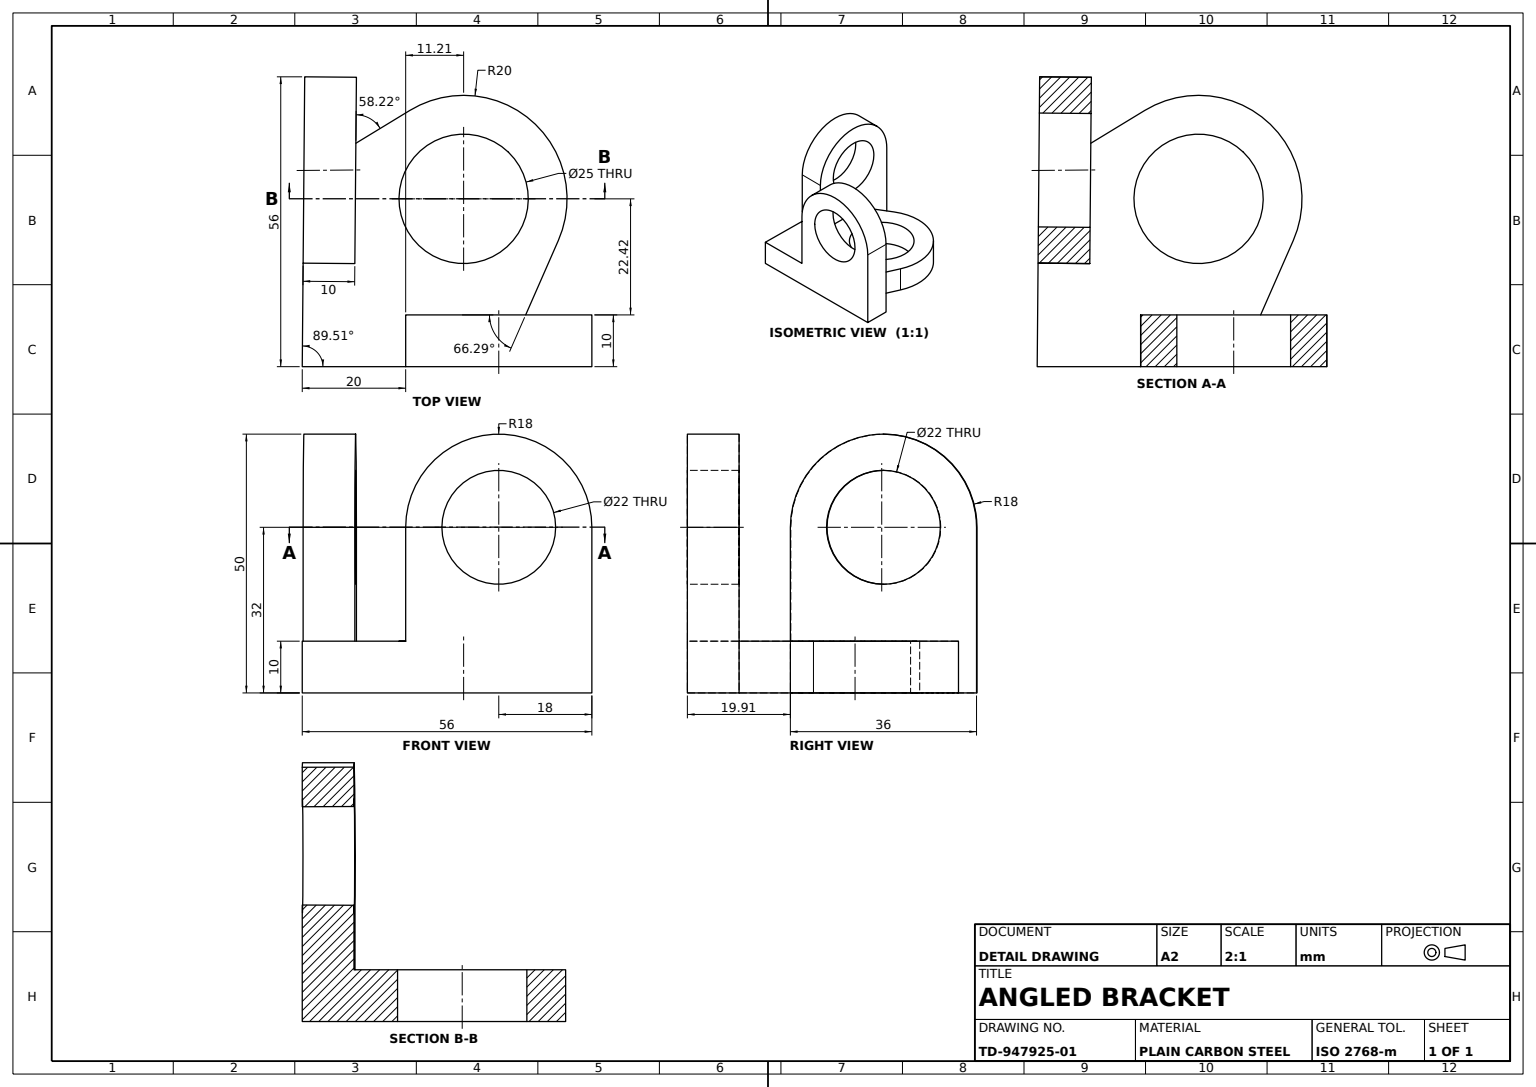
SolidWorks part; units mm, degrees
material "Plain Carbon Steel"
ref_plane "Front Plane" through (0, 0, 0) normal (0, 0, 1) x (1, 0, 0)
ref_plane "Top Plane" through (0, 0, 0) normal (0, 1, 0) x (1, 0, 0)
ref_plane "Right Plane" through (0, 0, 0) normal (1, 0, 0) x (0, 0, -1)
sketch "Base Plate Sketch" plane through (0, 0, 0) normal (0, 1, 0) x (1, 0, 0)
  line L0 (-19.3362, -21.1719) -> (-25.4663, -44.3681)
  line L1 (18.7702, -19.377) -> (27.9636, -44.3681)
  line L2 (-25.4663, -44.3681) -> (0, -71.2819)
  line L3 (0, -71.2819) -> (27.9636, -44.3681)
  arc A0 (18.7702, -19.377) -> (-19.3362, -21.1719) centre (0, -26.2819) ccw
  circle A1 centre (0, -26.2819) radius 12.5
  dimension "D1" = 40
  dimension "D2" = 25
  dimension "D5" = 26.2819
  dimension "D3" = 35
  dimension "D4" = 45
  dimension "D6" = 18.0862
  dimension "D7" = 25.4663
extrude "Base Plate" add sketch "Base Plate Sketch" along normal blind 10
ref_plane "Lug 1 Plane" through (35.6149, 0, 37.0041) normal (0.6935, 0, 0.7205) x (0.7205, 0, -0.6935)
sketch "Lug 1 Sketch" plane through (35.6149, 0, 37.0041) normal (0.6935, 0, 0.7205) x (0.7205, 0, -0.6935)
  line L0 (-29.4306, 10) -> (-29.4306, 32)
  line L1 (-49.4306, 10) -> (-10.6193, 10) construction
  line L3 (-10.6193, 10) -> (0.087, 10) construction
  line L4 (6.5694, 10) -> (6.5694, 32)
  line L5 (-49.4306, 10) -> (-49.4306, 0) construction
  line L6 (-49.4306, 0) -> (-10.6193, 0) construction
  line L9 (-29.4306, 10) -> (-29.4306, 0)
  line L10 (-29.4306, 0) -> (6.5694, 0)
  line L11 (6.5694, 10) -> (6.5694, 0)
  arc A0 (6.5694, 32) -> (-29.4306, 32) centre (-11.4306, 32) ccw
  circle A1 centre (-11.4306, 32) radius 11
  dimension "D4" = 36
  dimension "D5" = 22
  dimension "D1" = 20
  dimension "D2" = 32
  dimension "D3" = 36
  dimension "D6" = 18
  dimension "D7" = 10
extrude "Lug 1" add sketch "Lug 1 Sketch" against normal blind 10
ref_plane "Lug 2 Plane" through (-35.5865, 0, 33.6726) normal (-0.7264, 0, 0.6873) x (0.6873, 0, 0.7264)
sketch "Lug 2 Sketch" plane through (-35.5865, 0, 33.6726) normal (-0.7264, 0, 0.6873) x (0.6873, 0, 0.7264)
  line L0 (31.7771, 32) -> (31.7771, 0)
  line L2 (14.7246, 0) -> (51.7771, 0) construction
  line L3 (31.7771, 0) -> (-4.2229, 0)
  line L4 (2.0888, 0) -> (14.7246, 0) construction
  line L5 (-4.2229, 0) -> (-4.2229, 32)
  line L6 (51.7771, 10) -> (51.7771, 0) construction
  circle A0 centre (13.7771, 32) radius 11
  arc A1 (31.7771, 32) -> (-4.2229, 32) centre (13.7771, 32) ccw
  dimension "D1" = 36
  dimension "D2" = 22
  dimension "D3" = 32
  dimension "D4" = 20
  dimension "D5" = 36
  dimension "D6" = 18
extrude "Lug 2" add sketch "Lug 2 Sketch" against normal blind 10
